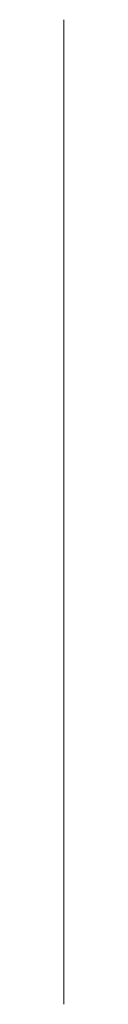
# Model space of a CAD drawing. Units: millimetres. Extents: x 574.2 to 592.2, y 785.6 to 810.6.
# Tile 1 of 1: x 592.2 to 592.2, y 797.61 to 810.61. Entities that reach past the tile are written whole.
import ezdxf

# ---------------------------------------------------------------- set-up
doc = ezdxf.new("R2010")
doc.units = ezdxf.units.MM
doc.layers.add('M-CONS', color=8, linetype='Continuous', lineweight=13)

msp = doc.modelspace()

# ---------------------------------------------------------------- linework, layer by layer
at = {"layer": 'M-CONS'}
for p, q in [((592.195, 810.61, 12), (592.195, 797.61, 12)), ((592.195, 797.61, 37), (592.195, 810.61, 37)), ((592.195, 810.61, 37), (592.195, 810.61, 49)), ((592.195, 810.61, 49), (592.195, 797.61, 49)), ((592.195, 797.61, 12), (592.195, 797.61, 37))]:
    msp.add_line(p, q, dxfattribs=at)

doc.saveas('drawing.dxf')
